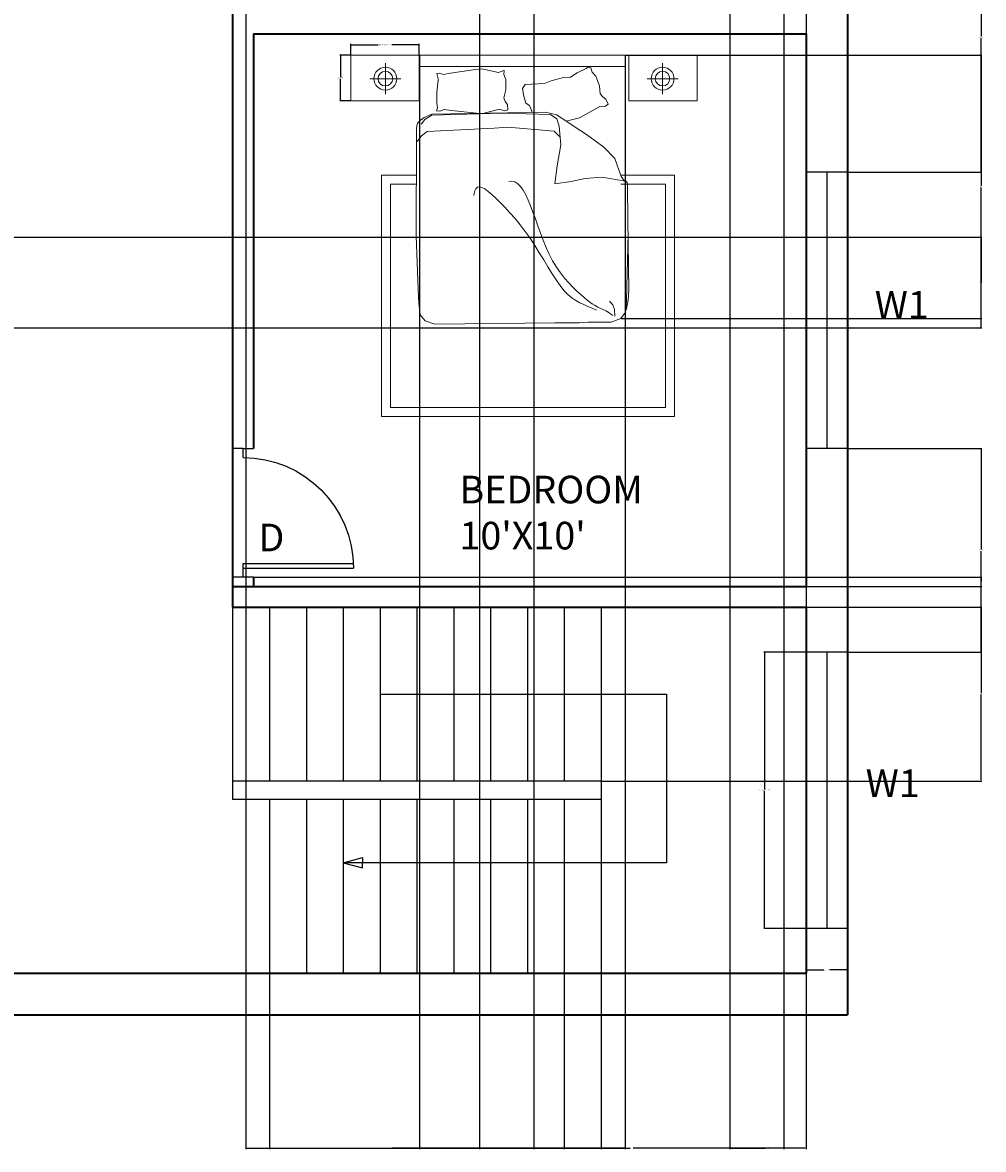
# Model space of a CAD drawing. Units: inches. Extents: x 3 to 420, y -502 to 54.
# Tile 3 of 6: x 212 to 420, y -502 to -257. Entities that reach past the tile are written whole.
import ezdxf

# ---------------------------------------------------------------- set-up
doc = ezdxf.new("R2010")
doc.units = ezdxf.units.IN
doc.header["$MEASUREMENT"] = 0
for name, color, linetype, lineweight in [('A-ANNO-DIMS', 2, 'Continuous', 18), ('A-ANNO-TEXT', 7, 'Continuous', 18), ('A-AREA-IDEN', 7, 'Continuous', 18), ('A-DOOR', 4, 'Continuous', 25), ('A-FLOR-STRS', 7, 'Continuous', 25), ('A-FURN', 8, 'Continuous', 18), ('A-GLAZ', 40, 'Continuous', 25), ('A-WALL', 7, 'Continuous', 35)]:
    doc.layers.add(name, color=color, linetype=linetype, lineweight=lineweight)
doc.styles.get("Standard").update_dxf_attribs({"font": 'arial.ttf'})
doc.dimstyles.get("Standard").update_dxf_attribs({"dimtxt": 0.18, "dimasz": 0.18, "dimexe": 0.18, "dimexo": 0.0625, "dimgap": 0.09, "dimtad": 0, "dimtih": 1, "dimtoh": 1, "dimdec": 0, "dimzin": 0, "dimdsep": 46, "dimlunit": 3, "dimtxsty": 'Standard', "dimcen": 0.09, "dimadec": 0, "dimazin": 0, "dimtfac": 1, "dimtdec": 0, "dimtofl": 0, "dimtmove": 0, "dimatfit": 3, "dimfxl": 1, "dimtolj": 1, "dimtzin": 0, "dimarcsym": 0})

# ---------------------------------------------------------------- blocks, each defined once
blk = doc.blocks.new('DOOR-SWING-24')
for p, q in [((2, 2.25), (2, 26.25)), ((3, 2.25), (3, 26.25)), ((0, 4.5), (0, 0)), ((28, 2.25), (28, 4.5)), ((0, 2.25), (2, 2.25)), ((2, 2.25), (3, 2.25)), ((26, 2.25), (28, 2.25)), ((28, 2.25), (28, 0))]:
    blk.add_line(p, q)
blk.add_arc((2, 2.25), 24, 0, 90)
blk = doc.blocks.new('WIN-W1-60')
for p, q in [((0, 9), (60, 9)), ((0, 9), (0, 0)), ((60, 9), (60, 0)), ((0, 4.5), (60, 4.5)), ((0, 0), (60, 0))]:
    blk.add_line(p, q)
blk = doc.blocks.new('NIGHTSTAND-SMALL')
for p, q in [((7.52, 8.16), (7.52, 1.41)), ((4.14, 4.79), (10.89, 4.79))]:
    blk.add_line(p, q)
blk.add_lwpolyline([(0, 0), (14.88, 0), (14.88, 9.92), (0, 9.92)], close=True)
for radius in [2.48, 1.59]:
    blk.add_circle((7.52, 4.79), radius)
blk = doc.blocks.new('*D15')
at = {"layer": 'A-ANNO-DIMS', "color": 0, "lineweight": -2, "transparency": 16777216}
for p, q in [((381.83, -393.71), (372.71, -393.71)), ((372.89, -393.89), (372.89, -423.52)), ((372.89, -453.53), (372.89, -423.89)), ((381.83, -453.71), (372.71, -453.71))]:
    blk.add_line(p, q, dxfattribs=at)
at = {"layer": 'A-ANNO-DIMS', "color": 0, "transparency": 16777216}
for points in [[(372.86, -393.89), (372.92, -393.89), (372.89, -393.71)], [(372.86, -453.53), (372.92, -453.53), (372.89, -453.71)]]:
    blk.add_solid(points, dxfattribs=at)
at = {"layer": 'Defpoints', "color": 0, "transparency": 16777216}
for p in [(381.89, -393.71), (372.89, -453.71), (381.89, -453.71)]:
    blk.add_point(p, dxfattribs=at)
at = {"layer": 'A-ANNO-DIMS', "color": 0, "transparency": 16777216, "insert": (372.89, -423.71), "char_height": 0.18, "attachment_point": 5}
blk.add_mtext('\\A1;WINDOW W1 5\'-0" TYP.', dxfattribs=at)
blk = doc.blocks.new('*D16')
at = {"layer": 'A-ANNO-DIMS', "color": 0, "lineweight": -2, "transparency": 16777216}
for p, q in [((381.89, -453.77), (381.89, -462.89)), ((390.89, -453.77), (390.89, -462.89)), ((382.07, -462.71), (385.75, -462.71)), ((390.71, -462.71), (387.03, -462.71))]:
    blk.add_line(p, q, dxfattribs=at)
at = {"layer": 'A-ANNO-DIMS', "color": 0, "transparency": 16777216}
for points in [[(382.07, -462.68), (382.07, -462.74), (381.89, -462.71)], [(390.71, -462.68), (390.71, -462.74), (390.89, -462.71)]]:
    blk.add_solid(points, dxfattribs=at)
at = {"layer": 'Defpoints', "color": 0, "transparency": 16777216}
for p in [(381.89, -453.71), (390.89, -453.71), (390.89, -462.71)]:
    blk.add_point(p, dxfattribs=at)
at = {"layer": 'A-ANNO-DIMS', "color": 0, "transparency": 16777216, "insert": (386.39, -462.71), "char_height": 0.18, "attachment_point": 5}
blk.add_mtext('\\A1;0\'-9" TYP.', dxfattribs=at)
blk = doc.blocks.new('*D31')
at = {"layer": 'A-ANNO-DIMS', "color": 0, "lineweight": -2, "transparency": 16777216}
for p, q in [((283.04, -263.98), (283.04, -261.63)), ((283.22, -261.81), (288.99, -261.81)), ((297.74, -261.81), (291.97, -261.81)), ((297.92, -263.98), (297.92, -261.63))]:
    blk.add_line(p, q, dxfattribs=at)
at = {"layer": 'A-ANNO-DIMS', "color": 0, "transparency": 16777216}
for points in [[(283.22, -261.78), (283.22, -261.84), (283.04, -261.81)], [(297.74, -261.78), (297.74, -261.84), (297.92, -261.81)]]:
    blk.add_solid(points, dxfattribs=at)
at = {"layer": 'Defpoints', "color": 0, "transparency": 16777216}
for p in [(297.92, -261.81), (283.04, -264.04), (297.92, -264.04)]:
    blk.add_point(p, dxfattribs=at)
at = {"layer": 'A-ANNO-DIMS', "color": 0, "transparency": 16777216, "insert": (290.48, -261.81), "char_height": 0.18, "attachment_point": 5}
blk.add_mtext('\\A1;NIGHTSTAND 1\'-3" TYP.', dxfattribs=at)
blk = doc.blocks.new('*D32')
at = {"layer": 'A-ANNO-DIMS', "color": 0, "lineweight": -2, "transparency": 16777216}
for p, q in [((282.98, -264.04), (280.63, -264.04)), ((280.81, -264.22), (280.81, -268.82)), ((280.81, -273.78), (280.81, -269.19)), ((282.98, -273.96), (280.63, -273.96))]:
    blk.add_line(p, q, dxfattribs=at)
at = {"layer": 'A-ANNO-DIMS', "color": 0, "transparency": 16777216}
for points in [[(280.78, -264.22), (280.84, -264.22), (280.81, -264.04)], [(280.78, -273.78), (280.84, -273.78), (280.81, -273.96)]]:
    blk.add_solid(points, dxfattribs=at)
at = {"layer": 'Defpoints', "color": 0, "transparency": 16777216}
for p in [(280.81, -264.04), (283.04, -264.04), (283.04, -273.96)]:
    blk.add_point(p, dxfattribs=at)
at = {"layer": 'A-ANNO-DIMS', "color": 0, "transparency": 16777216, "insert": (280.81, -269), "char_height": 0.18, "attachment_point": 5}
blk.add_mtext('\\A1;0\'-10" TYP.', dxfattribs=at)
blk = doc.blocks.new('*D51')
at = {"layer": 'A-ANNO-DIMS', "color": 0, "lineweight": -2, "transparency": 16777216}
for p, q in [((265.39, -463.52), (265.39, -501.64)), ((337.39, -463.52), (337.39, -501.64)), ((265.57, -501.46), (301.06, -501.46)), ((337.21, -501.46), (301.72, -501.46))]:
    blk.add_line(p, q, dxfattribs=at)
at = {"layer": 'A-ANNO-DIMS', "color": 0, "transparency": 16777216}
for points in [[(265.57, -501.43), (265.57, -501.49), (265.39, -501.46)], [(337.21, -501.43), (337.21, -501.49), (337.39, -501.46)]]:
    blk.add_solid(points, dxfattribs=at)
at = {"layer": 'Defpoints', "color": 0, "transparency": 16777216}
for p in [(265.39, -463.46), (337.39, -463.46), (337.39, -501.46)]:
    blk.add_point(p, dxfattribs=at)
at = {"layer": 'A-ANNO-DIMS', "color": 0, "transparency": 16777216, "insert": (301.39, -501.46), "char_height": 0.18, "attachment_point": 5}
blk.add_mtext('\\A1;6\'-0"', dxfattribs=at)
blk = doc.blocks.new('*D52')
at = {"layer": 'A-ANNO-DIMS', "color": 0, "lineweight": -2, "transparency": 16777216}
for p, q in [((337.45, -383.96), (420.07, -383.96)), ((419.89, -384.14), (419.89, -402.65)), ((419.89, -421.53), (419.89, -403.01)), ((337.45, -421.71), (420.07, -421.71))]:
    blk.add_line(p, q, dxfattribs=at)
at = {"layer": 'A-ANNO-DIMS', "color": 0, "transparency": 16777216}
for points in [[(419.86, -384.14), (419.92, -384.14), (419.89, -383.96)], [(419.86, -421.53), (419.92, -421.53), (419.89, -421.71)]]:
    blk.add_solid(points, dxfattribs=at)
at = {"layer": 'Defpoints', "color": 0, "transparency": 16777216}
for p in [(337.39, -383.96), (337.39, -421.71), (419.89, -421.71)]:
    blk.add_point(p, dxfattribs=at)
at = {"layer": 'A-ANNO-DIMS', "color": 0, "transparency": 16777216, "insert": (419.89, -402.83), "char_height": 0.18, "attachment_point": 5}
blk.add_mtext('\\A1;3\'-2"', dxfattribs=at)
blk = doc.blocks.new('*D53')
at = {"layer": 'A-ANNO-DIMS', "color": 0, "lineweight": -2, "transparency": 16777216}
for p, q in [((329.39, -463.52), (329.39, -501.64)), ((337.39, -463.52), (337.39, -501.64)), ((329.57, -501.46), (333.06, -501.46)), ((337.21, -501.46), (333.72, -501.46))]:
    blk.add_line(p, q, dxfattribs=at)
at = {"layer": 'A-ANNO-DIMS', "color": 0, "transparency": 16777216}
for points in [[(329.57, -501.43), (329.57, -501.49), (329.39, -501.46)], [(337.21, -501.43), (337.21, -501.49), (337.39, -501.46)]]:
    blk.add_solid(points, dxfattribs=at)
at = {"layer": 'Defpoints', "color": 0, "transparency": 16777216}
for p in [(329.39, -463.46), (337.39, -463.46), (337.39, -501.46)]:
    blk.add_point(p, dxfattribs=at)
at = {"layer": 'A-ANNO-DIMS', "color": 0, "transparency": 16777216, "insert": (333.39, -501.46), "char_height": 0.18, "attachment_point": 5}
blk.add_mtext('\\A1;0\'-8"', dxfattribs=at)
blk = doc.blocks.new('*D57')
at = {"layer": 'A-ANNO-DIMS', "color": 0, "lineweight": -2, "transparency": 16777216}
for p, q in [((390.95, -230.96), (420.07, -230.96)), ((419.89, -231.14), (419.89, -260.02)), ((419.89, -289.28), (419.89, -260.39)), ((390.95, -289.46), (420.07, -289.46))]:
    blk.add_line(p, q, dxfattribs=at)
at = {"layer": 'A-ANNO-DIMS', "color": 0, "transparency": 16777216}
for points in [[(419.86, -231.14), (419.92, -231.14), (419.89, -230.96)], [(419.86, -289.28), (419.92, -289.28), (419.89, -289.46)]]:
    blk.add_solid(points, dxfattribs=at)
at = {"layer": 'Defpoints', "color": 0, "transparency": 16777216}
for p in [(390.89, -230.96), (390.89, -289.46), (419.89, -289.46)]:
    blk.add_point(p, dxfattribs=at)
at = {"layer": 'A-ANNO-DIMS', "color": 0, "transparency": 16777216, "insert": (419.89, -260.21), "char_height": 0.18, "attachment_point": 5}
blk.add_mtext('\\A1;4\'-10 1/2"', dxfattribs=at)
blk = doc.blocks.new('*D58')
at = {"layer": 'A-ANNO-DIMS', "color": 0, "lineweight": -2, "transparency": 16777216}
for p, q in [((390.95, -349.46), (420.07, -349.46)), ((419.89, -349.64), (419.89, -371.4)), ((419.89, -393.53), (419.89, -371.76)), ((390.95, -393.71), (420.07, -393.71))]:
    blk.add_line(p, q, dxfattribs=at)
at = {"layer": 'A-ANNO-DIMS', "color": 0, "transparency": 16777216}
for points in [[(419.86, -349.64), (419.92, -349.64), (419.89, -349.46)], [(419.86, -393.53), (419.92, -393.53), (419.89, -393.71)]]:
    blk.add_solid(points, dxfattribs=at)
at = {"layer": 'Defpoints', "color": 0, "transparency": 16777216}
for p in [(390.89, -349.46), (390.89, -393.71), (419.89, -393.71)]:
    blk.add_point(p, dxfattribs=at)
at = {"layer": 'A-ANNO-DIMS', "color": 0, "transparency": 16777216, "insert": (419.89, -371.58), "char_height": 0.18, "attachment_point": 5}
blk.add_mtext('\\A1;3\'-8 1/2"', dxfattribs=at)
blk = doc.blocks.new('*D65')
at = {"layer": 'A-ANNO-DIMS', "color": 0, "lineweight": -2, "transparency": 16777216}
for p, q in [((260.22, -10.97), (260.22, -501.64)), ((322.8, -10.97), (322.8, -501.64)), ((260.4, -501.46), (290.97, -501.46)), ((322.62, -501.46), (292.05, -501.46))]:
    blk.add_line(p, q, dxfattribs=at)
at = {"layer": 'A-ANNO-DIMS', "color": 0, "transparency": 16777216}
for points in [[(260.4, -501.43), (260.4, -501.49), (260.22, -501.46)], [(322.62, -501.43), (322.62, -501.49), (322.8, -501.46)]]:
    blk.add_solid(points, dxfattribs=at)
at = {"layer": 'Defpoints', "color": 0, "transparency": 16777216}
for p in [(260.22, -10.9), (322.8, -10.9), (322.8, -501.46)]:
    blk.add_point(p, dxfattribs=at)
at = {"layer": 'A-ANNO-DIMS', "color": 0, "transparency": 16777216, "insert": (291.51, -501.46), "char_height": 0.18, "attachment_point": 5}
blk.add_mtext('\\A1;5\'-2 1/2"', dxfattribs=at)
blk = doc.blocks.new('*D67')
at = {"layer": 'A-ANNO-DIMS', "color": 0, "lineweight": -2, "transparency": 16777216}
for p, q in [((297.98, -264.1), (297.98, -501.64)), ((342.64, -264.1), (342.64, -501.64)), ((298.16, -501.46), (319.77, -501.46)), ((342.46, -501.46), (320.85, -501.46))]:
    blk.add_line(p, q, dxfattribs=at)
at = {"layer": 'A-ANNO-DIMS', "color": 0, "transparency": 16777216}
for points in [[(298.16, -501.43), (298.16, -501.49), (297.98, -501.46)], [(342.46, -501.43), (342.46, -501.49), (342.64, -501.46)]]:
    blk.add_solid(points, dxfattribs=at)
at = {"layer": 'Defpoints', "color": 0, "transparency": 16777216}
for p in [(297.98, -264.04), (342.64, -264.04), (342.64, -501.46)]:
    blk.add_point(p, dxfattribs=at)
at = {"layer": 'A-ANNO-DIMS', "color": 0, "transparency": 16777216, "insert": (320.31, -501.46), "char_height": 0.18, "attachment_point": 5}
blk.add_mtext('\\A1;3\'-8 1/2"', dxfattribs=at)
blk = doc.blocks.new('*D68')
at = {"layer": 'A-ANNO-DIMS', "color": 0, "lineweight": -2, "transparency": 16777216}
for p, q in [((342.7, -264.04), (420.07, -264.04)), ((419.89, -264.22), (419.89, -292.47)), ((419.89, -321.09), (419.89, -292.84)), ((341.72, -321.27), (420.07, -321.27))]:
    blk.add_line(p, q, dxfattribs=at)
at = {"layer": 'A-ANNO-DIMS', "color": 0, "transparency": 16777216}
for points in [[(419.86, -264.22), (419.92, -264.22), (419.89, -264.04)], [(419.86, -321.09), (419.92, -321.09), (419.89, -321.27)]]:
    blk.add_solid(points, dxfattribs=at)
at = {"layer": 'Defpoints', "color": 0, "transparency": 16777216}
for p in [(342.64, -264.04), (341.66, -321.27), (419.89, -321.27)]:
    blk.add_point(p, dxfattribs=at)
at = {"layer": 'A-ANNO-DIMS', "color": 0, "transparency": 16777216, "insert": (419.89, -292.65), "char_height": 0.18, "attachment_point": 5}
blk.add_mtext('\\A1;4\'-9"', dxfattribs=at)
blk = doc.blocks.new('*D69')
at = {"layer": 'A-ANNO-DIMS', "color": 0, "lineweight": -2, "transparency": 16777216}
for p, q in [((310.96, -174.99), (310.96, -501.64)), ((377.04, -174.99), (377.04, -501.64)), ((311.14, -501.46), (343.67, -501.46)), ((376.86, -501.46), (344.33, -501.46))]:
    blk.add_line(p, q, dxfattribs=at)
at = {"layer": 'A-ANNO-DIMS', "color": 0, "transparency": 16777216}
for points in [[(311.14, -501.43), (311.14, -501.49), (310.96, -501.46)], [(376.86, -501.43), (376.86, -501.49), (377.04, -501.46)]]:
    blk.add_solid(points, dxfattribs=at)
at = {"layer": 'Defpoints', "color": 0, "transparency": 16777216}
for p in [(310.96, -174.93), (377.04, -174.93), (377.04, -501.46)]:
    blk.add_point(p, dxfattribs=at)
at = {"layer": 'A-ANNO-DIMS', "color": 0, "transparency": 16777216, "insert": (344, -501.46), "char_height": 0.18, "attachment_point": 5}
blk.add_mtext('\\A1;5\'-6"', dxfattribs=at)
blk = doc.blocks.new('*D74')
at = {"layer": 'A-ANNO-DIMS', "color": 0, "lineweight": -2, "transparency": 16777216}
for p, q in [((102.86, -303.61), (420.07, -303.61)), ((419.89, -303.79), (419.89, -313.28)), ((419.89, -323.13), (419.89, -313.64)), ((102.86, -323.31), (420.07, -323.31))]:
    blk.add_line(p, q, dxfattribs=at)
at = {"layer": 'A-ANNO-DIMS', "color": 0, "transparency": 16777216}
for points in [[(419.86, -303.79), (419.92, -303.79), (419.89, -303.61)], [(419.86, -323.13), (419.92, -323.13), (419.89, -323.31)]]:
    blk.add_solid(points, dxfattribs=at)
at = {"layer": 'Defpoints', "color": 0, "transparency": 16777216}
for p in [(102.8, -303.61), (102.8, -323.31), (419.89, -323.31)]:
    blk.add_point(p, dxfattribs=at)
at = {"layer": 'A-ANNO-DIMS', "color": 0, "transparency": 16777216, "insert": (419.89, -313.46), "char_height": 0.18, "attachment_point": 5}
blk.add_mtext('\\A1;1\'-7 1/2"', dxfattribs=at)
blk = doc.blocks.new('*D77')
at = {"layer": 'A-ANNO-DIMS', "color": 0, "lineweight": -2, "transparency": 16777216}
for p, q in [((365.32, -254.98), (365.32, -501.64)), ((381.89, -255.02), (381.89, -501.64)), ((365.5, -501.46), (373.07, -501.46)), ((381.71, -501.46), (374.14, -501.46))]:
    blk.add_line(p, q, dxfattribs=at)
at = {"layer": 'A-ANNO-DIMS', "color": 0, "transparency": 16777216}
for points in [[(365.5, -501.43), (365.5, -501.49), (365.32, -501.46)], [(381.71, -501.43), (381.71, -501.49), (381.89, -501.46)]]:
    blk.add_solid(points, dxfattribs=at)
at = {"layer": 'Defpoints', "color": 0, "transparency": 16777216}
for p in [(365.32, -254.92), (381.89, -254.96), (381.89, -501.46)]:
    blk.add_point(p, dxfattribs=at)
at = {"layer": 'A-ANNO-DIMS', "color": 0, "transparency": 16777216, "insert": (373.6, -501.46), "char_height": 0.18, "attachment_point": 5}
blk.add_mtext('\\A1;1\'-4 1/2"', dxfattribs=at)
blk = doc.blocks.new('*D82')
at = {"layer": 'A-ANNO-DIMS', "color": 0, "lineweight": -2, "transparency": 16777216}
for p, q in [((261.95, -377.46), (420.07, -377.46)), ((419.89, -377.64), (419.89, -378.27)), ((419.89, -379.28), (419.89, -378.64)), ((261.95, -379.46), (420.07, -379.46))]:
    blk.add_line(p, q, dxfattribs=at)
at = {"layer": 'A-ANNO-DIMS', "color": 0, "transparency": 16777216}
for points in [[(419.86, -377.64), (419.92, -377.64), (419.89, -377.46)], [(419.86, -379.28), (419.92, -379.28), (419.89, -379.46)]]:
    blk.add_solid(points, dxfattribs=at)
at = {"layer": 'Defpoints', "color": 0, "transparency": 16777216}
for p in [(261.89, -377.46), (261.89, -379.46), (419.89, -379.46)]:
    blk.add_point(p, dxfattribs=at)
at = {"layer": 'A-ANNO-DIMS', "color": 0, "transparency": 16777216, "insert": (419.89, -378.46), "char_height": 0.18, "attachment_point": 5}
blk.add_mtext('\\A1;0\'-2"', dxfattribs=at)

msp = doc.modelspace()

# ---------------------------------------------------------------- linework, layer by layer
at = {"layer": 'A-FLOR-STRS'}
for p, q in [((257.39, -383.96), (257.39, -425.71)), ((265.39, -383.96), (265.39, -421.71)), ((273.39, -383.96), (273.39, -421.71)), ((281.39, -383.96), (281.39, -421.71)), ((289.39, -383.96), (289.39, -421.71)), ((297.39, -383.96), (297.39, -421.71)), ((305.39, -383.96), (305.39, -421.71)), ((313.39, -383.96), (313.39, -421.71)), ((321.39, -383.96), (321.39, -421.71)), ((329.39, -383.96), (329.39, -421.71)), ((337.39, -383.96), (337.39, -463.46)), ((289.39, -402.83), (351.6, -402.83)), ((351.6, -402.83), (351.6, -439.45)), ((337.39, -421.71), (257.39, -421.71)), ((337.39, -425.71), (257.39, -425.71)), ((265.39, -425.71), (265.39, -463.46)), ((273.39, -425.71), (273.39, -463.46)), ((281.39, -425.71), (281.39, -463.46)), ((289.39, -425.71), (289.39, -463.46)), ((297.39, -425.71), (297.39, -463.46)), ((305.39, -425.71), (305.39, -463.46)), ((313.39, -425.71), (313.39, -463.46)), ((321.39, -425.71), (321.39, -463.46)), ((329.39, -425.71), (329.39, -463.46)), ((281.39, -439.45), (285.62, -438.32)), ((351.6, -439.45), (281.39, -439.45)), ((281.39, -439.45), (285.62, -440.58)), ((285.62, -438.32), (285.62, -439.45)), ((285.62, -440.58), (285.62, -439.45))]:
    msp.add_line(p, q, dxfattribs=at)
at = {"layer": 'A-FURN'}
for p, q in [((297.98, -278.4), (297.98, -264.04)), ((302.09, -269.5), (301.7, -268.06)), ((311.47, -267.05), (310.12, -267.19)), ((315.13, -267.81), (311.47, -267.05)), ((316.26, -267.39), (315.13, -267.81)), ((316.36, -267.42), (316.26, -267.39)), ((316.36, -267.42), (316.28, -268.26)), ((316.36, -267.42), (316.28, -268.26)), ((316.28, -268.26), (316.73, -269.33)), ((326.52, -269.67), (329.21, -268.95)), ((329.21, -268.95), (330.78, -268.82)), ((330.78, -268.82), (332.17, -267.89)), ((330.78, -268.82), (332.17, -267.89)), ((332.17, -267.89), (334.14, -266.97)), ((335.48, -267.74), (336.27, -268.61)), ((336.27, -268.61), (337.02, -270.76)), ((316.71, -271.62), (316.3, -273.3)), ((316.73, -269.33), (316.71, -271.62)), ((320.91, -270.45), (325.1, -270.2)), ((325.1, -270.2), (326.52, -269.67)), ((337.02, -270.76), (337.21, -272.49)), ((316.3, -273.3), (316.58, -274.11)), ((316.58, -274.11), (317.08, -274.76)), ((337.21, -272.49), (337.75, -273.15)), ((337.75, -273.15), (338.43, -273.59)), ((338.43, -273.59), (338.91, -274.69)), ((315.31, -275.82), (311.69, -276.74)), ((316.45, -276.18), (315.31, -275.82)), ((317.15, -275.95), (316.45, -276.18)), ((317.08, -274.76), (317.15, -275.95)), ((337.12, -275.19), (332.72, -277.66)), ((338.32, -275.14), (337.12, -275.19)), ((338.91, -274.69), (338.32, -275.14)), ((297.35, -279.38), (297.28, -280.07)), ((297.28, -280.07), (297.31, -281.69)), ((297.31, -281.69), (297.22, -303.31)), ((342.56, -291.44), (342.65, -291.4)), ((343.23, -299.76), (343.15, -292.74)), ((343.38, -315.11), (343.23, -299.76)), ((297.22, -303.31), (297.68, -314.9)), ((343.28, -302.77), (342.98, -314.37)), ((297.68, -314.9), (297.84, -317.93)), ((342.98, -314.37), (342.91, -317.4)), ((343.26, -317.24), (343.38, -315.11)), ((297.84, -317.93), (298.12, -320.43)), ((339.96, -318.26), (339.24, -317.5)), ((342.91, -317.4), (342.71, -319.91)), ((342.84, -319.45), (343.26, -317.24)), ((298.12, -320.43), (299.21, -321.75)), ((340.29, -319.28), (339.96, -318.26)), ((340.36, -320.75), (340.29, -319.28)), ((342.71, -319.91), (341.66, -321.27)), ((299.21, -321.75), (301.32, -322.46)), ((327.38, -322.18), (301.32, -322.46)), ((327.38, -322.18), (332.71, -322.18)), ((332.71, -322.18), (334.59, -322.04)), ((334.59, -322.04), (339.56, -322.04)), ((341.66, -321.27), (339.56, -322.04))]:
    msp.add_line(p, q, dxfattribs=at)
for points in [[(297.98, -264.04), (342.64, -264.04), (342.64, -291.36)], [(342.64, -266.52), (297.98, -266.52)], [(335.48, -267.74), (335.19, -266.83), (334.6, -266.64), (334.14, -266.97)], [(310.12, -267.19), (304.72, -268.01), (303.15, -268.27), (302.22, -267.97), (301.7, -268.06)], [(310.33, -276.65), (304.9, -276.08), (303.32, -275.89), (302.4, -276.23), (301.64, -276.13), (301.85, -275.53), (301.73, -274.5), (301.69, -272.11), (302.03, -269.5)], [(320.91, -270.45), (320.33, -271.28), (320.61, -273), (321.02, -274.52), (321.85, -275), (322.33, -276.24), (322.34, -276.47)], [(298.35, -278.13), (298.97, -277.6), (300.64, -276.9), (325.31, -276.41), (327.79, -277.05), (331.75, -279.68), (334.24, -281.32), (337.98, -284.07), (340.37, -286.51), (341.78, -290.41), (342.47, -291.43)], [(297.37, -279.34), (297.51, -278.87), (297.73, -278.52), (297.98, -278.4), (298.27, -278.14), (298.31, -278.12)], [(342.64, -291.46), (337.63, -290.59), (333.94, -290.87), (330.92, -291.47), (327.34, -291.98), (327.82, -288.07), (328.63, -283.52), (328.27, -279.51), (327.75, -277.89), (326.44, -276.96), (315.86, -276.67), (300.64, -277.12), (299.09, -278.04), (298.43, -278.95), (298.34, -279.04)], [(332.72, -277.66), (329.79, -278.38)], [(328.33, -281.73), (327.21, -280.58), (317.14, -279.73), (314.2, -279.9), (299.62, -280.63), (298.39, -281.56), (297.46, -282.8)], [(341.68, -290.13), (353.35, -290.13), (353.35, -342.57), (289.68, -342.57), (289.68, -290.13), (297.27, -290.13)], [(341.68, -292.11), (351.37, -292.11), (351.37, -340.58), (291.67, -340.58), (291.67, -292.11), (297.27, -292.11)], [(336.4, -319.42), (335.45, -319.01), (334.53, -318.62), (333.63, -318.24), (332.75, -317.83), (331.88, -317.35), (331.03, -316.77), (330.18, -316.06), (329.33, -315.18), (328.48, -314.12), (327.62, -312.89), (326.74, -311.52), (325.85, -310.06), (324.93, -308.53), (323.98, -306.96), (322.99, -305.38), (321.97, -303.83), (320.9, -302.34), (319.81, -300.91), (318.71, -299.57), (317.61, -298.31), (316.54, -297.14), (315.51, -296.09), (314.54, -295.15), (313.64, -294.33), (312.84, -293.65), (312.13, -293.13), (311.52, -292.79), (310.99, -292.65), (310.56, -292.74), (310.21, -293.07), (309.94, -293.67), (309.76, -294.56)], [(339.92, -320.59), (339.51, -320.28), (339.13, -320.02), (338.79, -319.8), (338.47, -319.62), (338.17, -319.47), (337.88, -319.34), (337.6, -319.21), (337.31, -319.08), (337.01, -318.95), (336.69, -318.79), (336.33, -318.59), (335.94, -318.35), (335.49, -318.06), (334.98, -317.69), (334.4, -317.24), (333.73, -316.71), (332.98, -316.06), (332.15, -315.32), (331.28, -314.47), (330.37, -313.53), (329.45, -312.48), (328.55, -311.33), (327.68, -310.09), (326.86, -308.75), (326.11, -307.31), (325.43, -305.81), (324.8, -304.27), (324.21, -302.7), (323.66, -301.15), (323.12, -299.63), (322.6, -298.17), (322.09, -296.79), (321.56, -295.53), (321.02, -294.4), (320.47, -293.42), (319.89, -292.62), (319.3, -292), (318.68, -291.6), (318.03, -291.42), (317.35, -291.5)], [(343.15, -292.68), (343.08, -291.71), (342.8, -291.42), (342.64, -291.36)]]:
    msp.add_lwpolyline(points, dxfattribs=at)
at = {"layer": 'A-WALL'}
for p, q in [((390.89, 4.54), (390.89, -472.46)), ((257.39, -254.96), (257.39, -383.96)), ((261.89, -259.46), (381.89, -259.46)), ((261.89, -259.46), (261.89, -349.46)), ((381.89, -259.46), (381.89, -379.46)), ((261.89, -377.46), (261.89, -379.46)), ((257.39, -379.46), (381.89, -379.46)), ((257.39, -383.96), (381.89, -383.96)), ((381.89, -383.96), (381.89, -463.46)), ((84.39, -463.46), (381.89, -463.46)), ((32.39, -472.46), (390.89, -472.46))]:
    msp.add_line(p, q, dxfattribs=at)

# ---------------------------------------------------------------- block references
at = {"layer": 'A-DOOR', "extrusion": (0, 0, -1), "zscale": -1, "rotation": 90.00000000000026}
msp.add_blockref('DOOR-SWING-24', (-257.39, -377.46), dxfattribs=at)
at = {"layer": 'A-FURN'}
msp.add_blockref('NIGHTSTAND-SMALL', (283.04, -273.96), dxfattribs=at)
at = {"layer": 'A-FURN', "extrusion": (0, 0, -1), "zscale": -1}
msp.add_blockref('NIGHTSTAND-SMALL', (-358.26, -273.96), dxfattribs=at)
at = {"layer": 'A-GLAZ', "rotation": 270}
for p in [(381.89, -289.46), (381.89, -393.71)]:
    msp.add_blockref('WIN-W1-60', p, dxfattribs=at)

# ---------------------------------------------------------------- texts
at = {"layer": 'A-ANNO-TEXT', "char_height": 6, "attachment_point": 1}
for s, insert in [('W1', (396.81, -315.28)), ('D', (262.99, -365.82)), ('W1', (394.85, -419.2))]:
    msp.add_mtext(s, dxfattribs=dict(at, insert=insert))
at = {"layer": 'A-AREA-IDEN', "insert": (306.64, -355.41), "char_height": 6, "attachment_point": 1}
msp.add_mtext("BEDROOM\\P10'X10'", dxfattribs=at)

# ---------------------------------------------------------------- dimensions: what is measured, and where the dimension line sits
at = {"layer": 'A-ANNO-DIMS'}
for base, p1, p2, picture, middle in [((322.8, -501.46), (260.22, -10.9), (322.8, -10.9), '*D65', (291.51, -501.46)), ((377.04, -501.46), (310.96, -174.93), (377.04, -174.93), '*D69', (344, -501.46)), ((381.89, -501.46), (365.32, -254.92), (381.89, -254.96), '*D77', (373.6, -501.46)), ((342.64, -501.46), (297.98, -264.04), (342.64, -264.04), '*D67', (320.31, -501.46)), ((337.39, -501.46), (265.39, -463.46), (337.39, -463.46), '*D51', (301.39, -501.46)), ((337.39, -501.46), (329.39, -463.46), (337.39, -463.46), '*D53', (333.39, -501.46))]:
    dim = msp.add_linear_dim(base=base, p1=p1, p2=p2, dimstyle='Standard', override={"dimdec": 1, "dimlfac": 1, "dimrnd": 0, "dimzin": 1, "dimdsep": 46, "dimlunit": 4, "dimfrac": 2}, dxfattribs=at)
    dim.commit()
    dim.dimension.update_dxf_attribs({"geometry": picture, "text_midpoint": middle})
for base, p1, p2, picture, middle in [((419.89, -289.46), (390.89, -230.96), (390.89, -289.46), '*D57', (419.89, -260.21)), ((419.89, -321.27), (342.64, -264.04), (341.66, -321.27), '*D68', (419.89, -292.65)), ((419.89, -323.31), (102.8, -303.61), (102.8, -323.31), '*D74', (419.89, -313.46)), ((419.889185, -393.706282), (390.889185, -349.456282), (390.889185, -393.706282), '*D58', (419.889185, -371.581282)), ((419.89, -379.46), (261.89, -377.46), (261.89, -379.46), '*D82', (419.89, -378.46)), ((419.889185, -421.706282), (337.389185, -383.956282), (337.389185, -421.706282), '*D52', (419.889185, -402.831282))]:
    dim = msp.add_linear_dim(base=base, p1=p1, p2=p2, angle=90, dimstyle='Standard', override={"dimdec": 1, "dimlfac": 1, "dimrnd": 0, "dimzin": 1, "dimdsep": 46, "dimlunit": 4, "dimfrac": 2}, dxfattribs=at)
    dim.commit()
    dim.dimension.update_dxf_attribs({"geometry": picture, "text_midpoint": middle})
for base, p1, p2, text, picture, middle in [((297.92, -261.81), (283.04, -264.04), (297.92, -264.04), 'NIGHTSTAND <> TYP.', '*D31', (290.48, -261.81)), ((390.89, -462.71), (381.89, -453.71), (390.89, -453.71), '<> TYP.', '*D16', (386.39, -462.71))]:
    dim = msp.add_linear_dim(base=base, p1=p1, p2=p2, text=text, dimstyle='Standard', override={"dimdec": 1, "dimlfac": 1, "dimrnd": 0, "dimzin": 1, "dimdsep": 46, "dimlunit": 4, "dimfrac": 2}, dxfattribs=at)
    dim.commit()
    dim.dimension.update_dxf_attribs({"geometry": picture, "text_midpoint": middle})
for base, p1, p2, angle, text, picture, middle in [((280.81, -264.04), (283.04, -273.96), (283.04, -264.04), 90, '<> TYP.', '*D32', (280.81, -269)), ((372.89, -453.71), (381.89, -393.71), (381.89, -453.71), 270, 'WINDOW W1 <> TYP.', '*D15', (372.89, -423.71))]:
    dim = msp.add_linear_dim(base=base, p1=p1, p2=p2, angle=angle, text=text, dimstyle='Standard', override={"dimdec": 1, "dimlfac": 1, "dimrnd": 0, "dimzin": 1, "dimdsep": 46, "dimlunit": 4, "dimfrac": 2}, dxfattribs=at)
    dim.commit()
    dim.dimension.update_dxf_attribs({"geometry": picture, "text_midpoint": middle})

doc.saveas('drawing.dxf')
